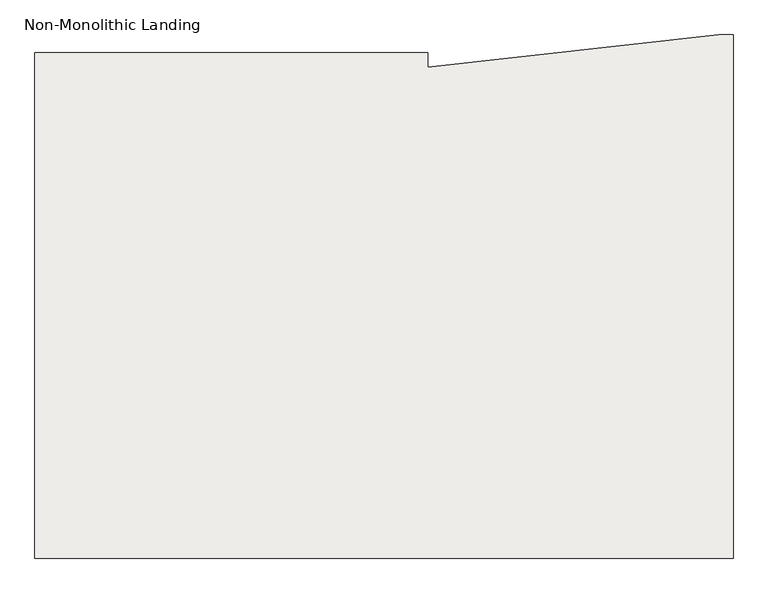
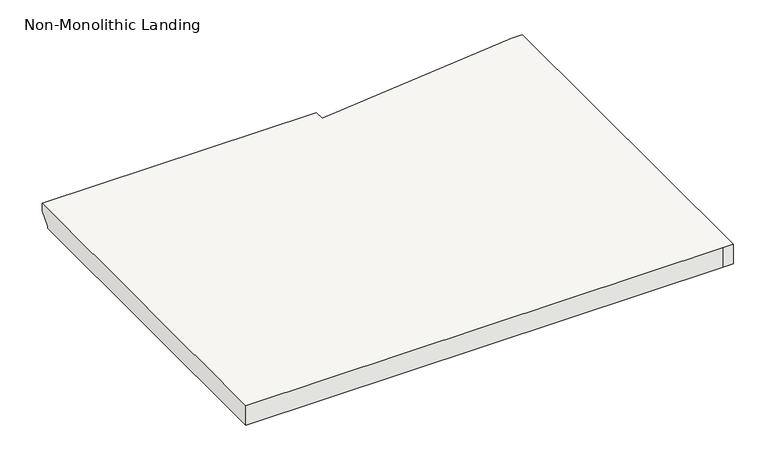
"""IFC4 building model written with IfcOpenShell, lengths in millimetres: slab geometry, Non-Monolithic Landing."""

from ifc_helpers import new_model, si_unit, origin, place, context, project, spatial, faceted_brep, source, transform, mapped, element, save


def non_monolithic_landing_a4a5f0de(model_context):
    return source(origin(), model_context, "Body", "Brep", [
        faceted_brep([(-10581.8342448, -2032.7993654, 5365.75), (-10581.8342448, -2032.7993654, 5384.8), (-10581.8342448, -2058.1993654, 5384.8), (-10581.8342448, -2058.1993654, 5340.35), (-11268.1522729, -2032.7993654, 5365.75), (-11268.1522729, -2032.7993654, 5384.8), (-11268.1522729, -2058.1993654, 5340.35), (-11268.1522729, -2916.0844117, 5384.8), (-10074.3522729, -2916.0844117, 5384.8), (-10048.9522729, -2916.0844117, 5384.8), (-10048.9522729, -2001.6844117, 5384.8), (-10074.3522729, -2001.6844117, 5384.8), (-11268.1522729, -2058.1993654, 5334.0), (-10581.8342448, -2058.1993654, 5334.0), (-10074.3522729, -2001.6844117, 5334.0), (-10048.9522729, -2001.6844117, 5334.0), (-10048.9522729, -2916.0844117, 5334.0), (-10074.3522729, -2916.0844117, 5334.0), (-11268.1522729, -2916.0844117, 5334.0)], [[[0, 1, 2, 3]], [[4, 5, 1, 0]], [[6, 4, 0, 3]], [[7, 8, 9, 10, 11, 2, 1, 5]], [[12, 13, 14, 15, 16, 17, 18]], [[13, 12, 6, 3]], [[7, 5, 4, 6, 12, 18]], [[8, 7, 18, 17]], [[9, 8, 17, 16]], [[10, 9, 16, 15]], [[11, 10, 15, 14]], [[2, 11, 14, 13, 3]]]),
    ])


if __name__ == "__main__":
    model = new_model("IFC4")
    model_context = context("Model", 3, world=origin())
    ifc_project = project(units=[si_unit("LENGTHUNIT", "METRE", prefix="MILLI")], contexts=[model_context])
    site = spatial("IfcSite", under=ifc_project)
    building = spatial("IfcBuilding", under=site)
    placement = place(None, origin())
    non_monolithic_landing_shape = non_monolithic_landing_a4a5f0de(model_context)
    element("IfcSlab", 1, ObjectType="Non-Monolithic Landing", at=placement, inside=building, context=model_context, shape_type="MappedRepresentation", body=[
        mapped(non_monolithic_landing_shape, transform((0.0, 0.0, 0.0), x_axis=(1.0, 0.0, 0.0), y_axis=(0.0, 1.0, 0.0), z_axis=(0.0, 0.0, 1.0))),
    ])
    save(model, "model.ifc")
